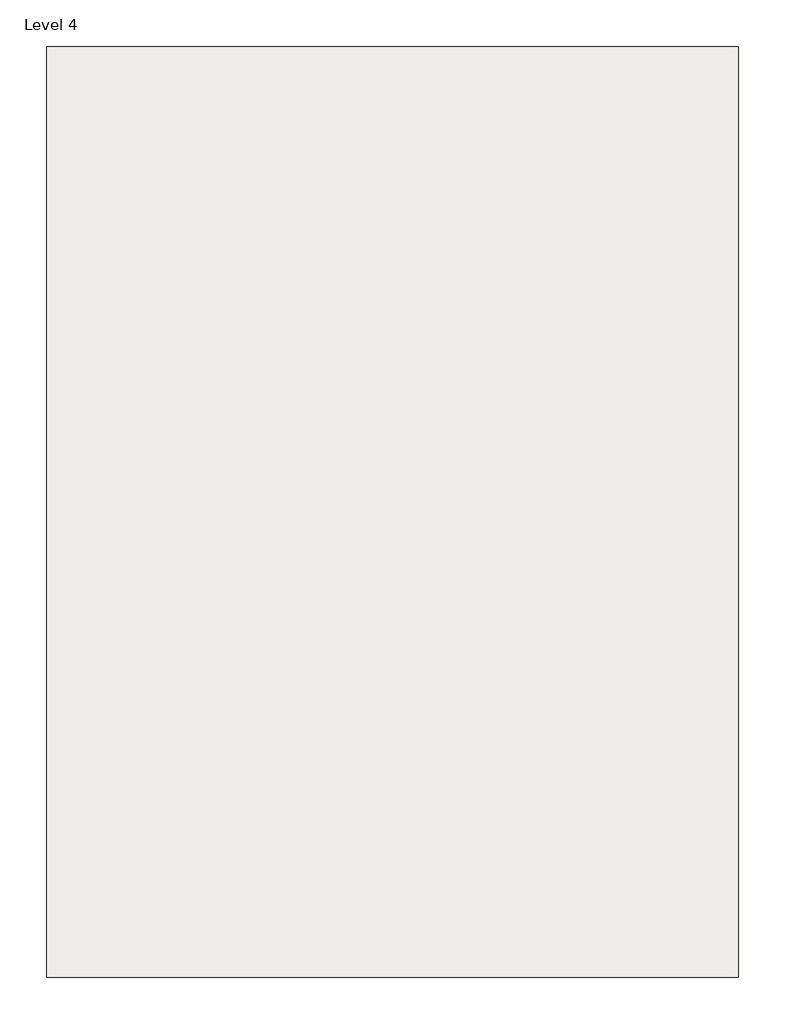
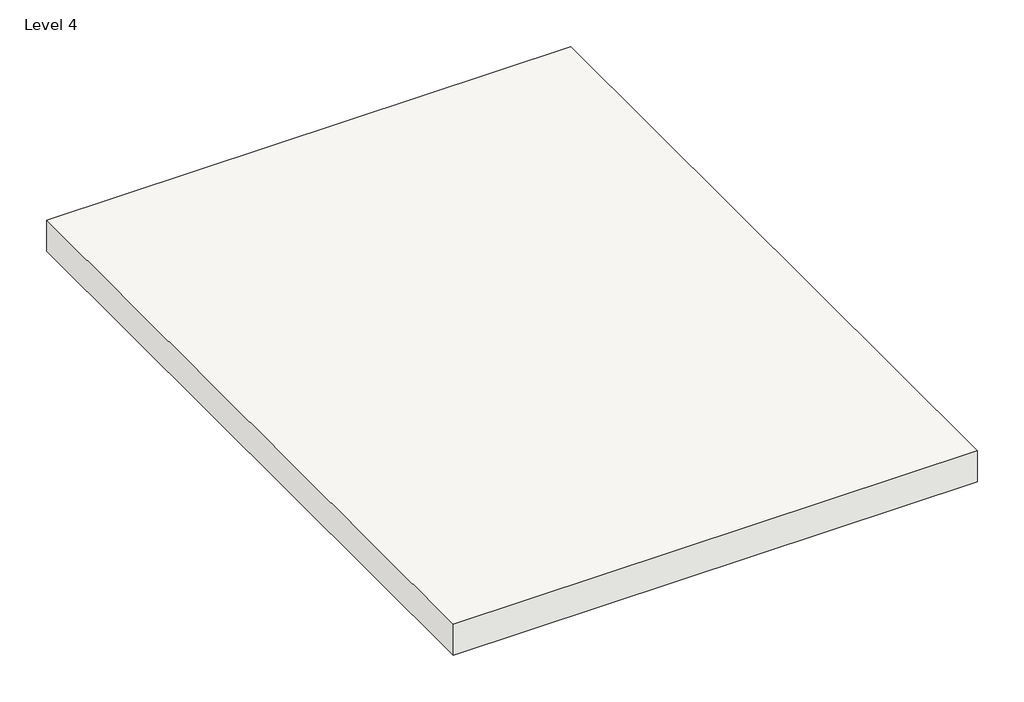
# One storey: 1 roof.
"""IFC4 building model written with IfcOpenShell, lengths in millimetres."""

from ifc_helpers import new_model, si_unit, frame, origin, place, context, project, spatial, polyline, outline, extrude, element, save

model = new_model("IFC4")

# Units and contexts
model_context = context("Model", 3, world=origin())
ifc_project = project(units=[si_unit("LENGTHUNIT", "METRE", prefix="MILLI")], contexts=[model_context])

# Site, building, storey
site = spatial("IfcSite", under=ifc_project)
building = spatial("IfcBuilding", under=site)
storey = spatial("IfcBuildingStorey", under=building, Name="Level 4", Elevation=10972.8)

# Roof
placement = place(None, origin())
element("IfcRoof", 1, ObjectType="Generic - 12\"", at=placement, inside=storey, context=model_context, shape_type="SweptSolid", body=[
    extrude(outline(polyline([(-7773.0932708, 232.3399767), (-12654.8431118, 232.3399767), (-12654.8431118, 6798.7609482), (-7773.0932708, 6798.7609482), (-7773.0932708, 232.3399767)])), frame((0.0, 0.0, 10363.2), z_axis=(0.0, 0.0, 1.0), x_axis=(1.0, 0.0, 0.0)), (0.0, 0.0, 1.0), 304.8),
])

save(model, "model.ifc")

# Revit data of these elements
# Type "Generic - 12\""
#   Assembly Code = "B1020"
#   Layers, outside or top first: 1' - 0" no material (function 1)
# Element 1 (IfcRoof, "Generic - 12\"")
#   built-in parameter 1001705 = 35 (stored number, unit not read)
#   built-in parameter 1001701 = -2 (stored number, unit not read)
#   built-in parameter 1001710 = 33615
#   Phase Created = New Construction
#   Materials on its faces: "Default Roof"
# Materials
#   "Default Roof": colour RGB 88 101 114, transparency 0
